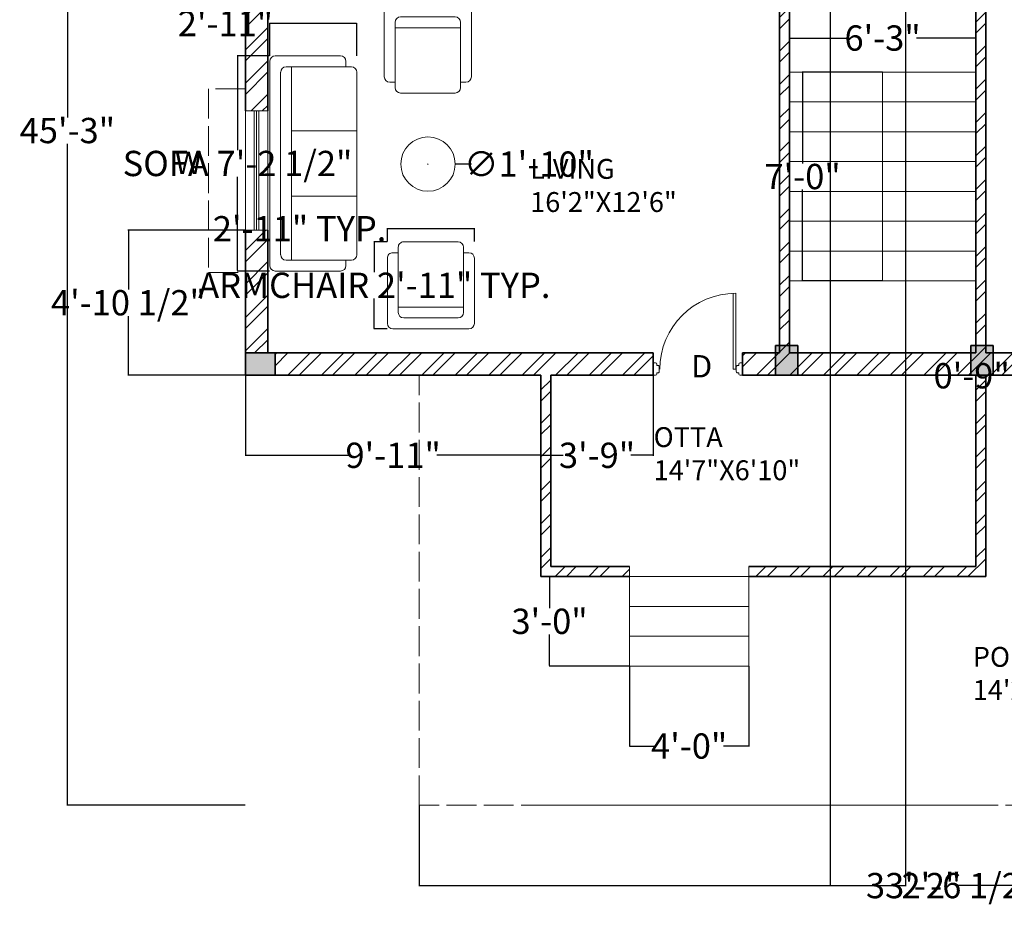
# Model space of a CAD drawing. Units: inches. Extents: x 2379 to 3013, y 1431 to 2110.
# Tile 1 of 10: x 2379 to 2775, y 1431 to 1795. Entities that reach past the tile are written whole.
import ezdxf

# ---------------------------------------------------------------- set-up
doc = ezdxf.new("R2010")
doc.units = ezdxf.units.IN
doc.linetypes.add('ACAD_ISO02W100', pattern=[15, 12, -3])
for name, color, linetype, lineweight in [('00 FURNITURE', 15, 'Continuous', 15), ('A-ANNO-DIMS', 2, 'Continuous', 18), ('A-ANNO-TEXT', 7, 'Continuous', 18), ('A-AREA-IDEN', 7, 'Continuous', 18), ('A-COLS', 7, 'Continuous', 35), ('A-COLS-PATT', 252, 'Continuous', 13), ('A-DOOR', 4, 'Continuous', 18), ('A-FLOR', 8, 'Continuous', 18), ('A-FLOR-STRS', 7, 'Continuous', 18), ('A-ROOF-OVHD', 11, 'ACAD_ISO02W100', 13), ('A-WALL-PATT', 8, 'Continuous', 13), ('WALL', 7, 'Continuous', 35), ('WINDOW', 4, 'Continuous', 15)]:
    doc.layers.add(name, color=color, linetype=linetype, lineweight=lineweight)
doc.styles.get("Standard").update_dxf_attribs({"font": 'arial.ttf'})
doc.dimstyles.get("Standard").update_dxf_attribs({"dimtxt": 10.18, "dimasz": 0.18, "dimexe": 0.18, "dimexo": 0.0625, "dimgap": 0.09, "dimtad": 0, "dimtih": 1, "dimtoh": 1, "dimdec": 0, "dimzin": 0, "dimdsep": 46, "dimlunit": 3, "dimtxsty": 'Standard', "dimcen": 0.09, "dimadec": 0, "dimazin": 0, "dimtfac": 1, "dimtdec": 0, "dimtofl": 0, "dimtmove": 0, "dimatfit": 3, "dimfxl": 1, "dimtolj": 1, "dimtzin": 0, "dimarcsym": 0})

# ---------------------------------------------------------------- blocks, each defined once
blk = doc.blocks.new('column')
for p, q in [((2588.21, 2021.79), (2597.21, 2021.79)), ((2588.21, 2009.79), (2588.21, 2021.79)), ((2597.21, 2021.79), (2597.21, 2009.79)), ((2597.21, 2009.79), (2588.21, 2009.79))]:
    blk.add_line(p, q)
blk = doc.blocks.new('DDD')
at = {"layer": '00 FURNITURE'}
for p, q in [((-12579.77, -15859.53), (-12579.77, -15829.05)), ((-12578.77, -15859.53), (-12578.77, -15829.03)), ((-12612.02, -15857.03), (-12612.02, -15862.03)), ((-12611.02, -15857.03), (-12612.02, -15857.03)), ((-12610.52, -15858.03), (-12610.52, -15857.53)), ((-12578.77, -15859.53), (-12579.77, -15859.53)), ((-12577.52, -15858.03), (-12577.52, -15857.53)), ((-12577.02, -15857.03), (-12576.02, -15857.03)), ((-12576.02, -15857.03), (-12576.02, -15862.03)), ((-12612.02, -15862.03), (-12611.02, -15862.03)), ((-12610.52, -15861.53), (-12610.52, -15861.03)), ((-12577.52, -15861.53), (-12577.52, -15861.03)), ((-12576.02, -15862.03), (-12577.02, -15862.03))]:
    blk.add_line(p, q, dxfattribs=at)
for points in [[(-12610.52, -15861.03), (-12610.02, -15861.03, 0.414214), (-12609.52, -15860.53), (-12609.52, -15858.53, 0.414214), (-12610.02, -15858.03), (-12610.52, -15858.03)], [(-12577.52, -15861.03), (-12578.02, -15861.03, -0.414214), (-12578.52, -15860.53), (-12578.52, -15858.53, -0.414214), (-12578.02, -15858.03), (-12577.52, -15858.03)]]:
    blk.add_lwpolyline(points, format="xyb", dxfattribs=at)
for centre, radius, start, end in [((-12578.77, -15859.53), 30.5, 90, 180), ((-12611.02, -15857.53), 0.5, 0, 90), ((-12577.02, -15857.53), 0.5, 90, 180), ((-12611.02, -15861.53), 0.5, 270, 0), ((-12577.02, -15861.53), 0.5, 180, 270)]:
    blk.add_arc(centre, radius, start, end, dxfattribs=at)
blk = doc.blocks.new('sofa 6')
for p, q in [((-1100, 167), (-1100, 834)), ((-1044, 890), (1044, 890)), ((1100, 834), (1100, 167)), ((-989, 56), (-989, 723)), ((-933, 779), (933, 779)), ((989, 723), (989, 56)), ((-989, 667), (989, 667)), ((-334, 667), (-334, 0)), ((334, 667), (334, 0)), ((-989, 111), (-1044, 111)), ((1044, 111), (989, 111)), ((933, 0), (-933, 0))]:
    blk.add_line(p, q)
for centre, start, end in [((-1044, 834), 90, 180), ((1044, 834), 0, 90), ((-933, 723), 90, 180), ((933, 723), 0, 90), ((-1044, 167), 180, 270), ((1044, 167), 270, 0), ((-933, 56), 180, 270), ((933, 56), 270, 0)]:
    blk.add_arc(centre, 55.6, start, end)
blk = doc.blocks.new('*D12')
at = {"layer": 'A-ANNO-DIMS', "color": 0, "lineweight": -2, "transparency": 16777216}
for p, q in [((2688.63, 1773.67), (2688.63, 1787.52)), ((2763.63, 1773.67), (2763.63, 1787.52)), ((2688.81, 1787.34), (2712.48, 1787.34)), ((2763.45, 1787.34), (2739.78, 1787.34))]:
    blk.add_line(p, q, dxfattribs=at)
at = {"layer": 'A-ANNO-DIMS', "color": 0, "transparency": 16777216}
for points in [[(2688.81, 1787.37), (2688.81, 1787.31), (2688.63, 1787.34)], [(2763.45, 1787.37), (2763.45, 1787.31), (2763.63, 1787.34)]]:
    blk.add_solid(points, dxfattribs=at)
at = {"layer": 'Defpoints', "color": 0, "transparency": 16777216}
for p in [(2763.63, 1787.34), (2688.63, 1773.61), (2763.63, 1773.61)]:
    blk.add_point(p, dxfattribs=at)
at = {"layer": 'A-ANNO-DIMS', "color": 0, "transparency": 16777216, "insert": (2726.13, 1787.34), "char_height": 10.18, "attachment_point": 5}
blk.add_mtext('\\A1;6\'-3"', dxfattribs=at)
blk = doc.blocks.new('*D13')
at = {"layer": 'A-ANNO-DIMS', "color": 0, "lineweight": -2, "transparency": 16777216}
for p, q in [((2469.57, 2021.61), (2397.82, 2021.61)), ((2398, 2021.43), (2398, 1755.4)), ((2398, 1478.79), (2398, 1744.82)), ((2469.57, 1478.61), (2397.82, 1478.61))]:
    blk.add_line(p, q, dxfattribs=at)
at = {"layer": 'A-ANNO-DIMS', "color": 0, "transparency": 16777216}
for points in [[(2397.97, 2021.43), (2398.03, 2021.43), (2398, 2021.61)], [(2397.97, 1478.79), (2398.03, 1478.79), (2398, 1478.61)]]:
    blk.add_solid(points, dxfattribs=at)
at = {"layer": 'Defpoints', "color": 0, "transparency": 16777216}
for p in [(2469.63, 2021.61), (2398, 1478.61), (2469.63, 1478.61)]:
    blk.add_point(p, dxfattribs=at)
at = {"layer": 'A-ANNO-DIMS', "color": 0, "transparency": 16777216, "insert": (2398, 1750.11), "char_height": 10.18, "attachment_point": 5}
blk.add_mtext('\\A1;45\'-3"', dxfattribs=at)
blk = doc.blocks.new('CHAIR-LOUNGE')
for p, q in [((0, 32.85), (0, 6.57)), ((32.85, 35.04), (2.19, 35.04)), ((35.04, 6.57), (35.04, 32.85)), ((4.38, 28.47), (4.38, 2.19)), ((28.47, 30.66), (6.57, 30.66)), ((30.66, 2.19), (30.66, 28.47)), ((30.66, 26.28), (4.38, 26.28)), ((2.19, 4.38), (4.38, 4.38)), ((30.66, 4.38), (32.85, 4.38)), ((6.57, 0), (28.47, 0))]:
    blk.add_line(p, q)
for centre, start, end in [((2.19, 32.85), 90, 180), ((32.85, 32.85), 0, 90), ((6.57, 28.47), 90, 180), ((28.47, 28.47), 0, 90), ((2.19, 6.57), 180, 270), ((32.85, 6.57), 270, 0), ((6.57, 2.19), 180, 270), ((28.47, 2.19), 270, 0)]:
    blk.add_arc(centre, 2.19, start, end)
blk = doc.blocks.new('WIN-48IN')
for p, q in [((0, 48), (0, 0)), ((9, 48), (0, 48)), ((3.5, 48), (3.5, 0)), ((4.5, 48), (4.5, 0)), ((5.5, 48), (5.5, 0)), ((9, 0), (9, 48)), ((9, 0), (0, 0))]:
    blk.add_line(p, q)
blk = doc.blocks.new('*D23')
at = {"layer": 'A-ANNO-DIMS', "color": 0, "lineweight": -2, "transparency": 16777216}
for p, q in [((2816.16, 1660.61), (2808.84, 1660.61)), ((2809.02, 1660.43), (2809.02, 1651.79)), ((2816.16, 1651.61), (2808.84, 1651.61)), ((2809.02, 1651.43), (2808.84, 1651.43)), ((2809.02, 1651.61), (2809.02, 1651.43))]:
    blk.add_line(p, q, dxfattribs=at)
at = {"layer": 'A-ANNO-DIMS', "color": 0, "transparency": 16777216}
for points in [[(2808.99, 1660.43), (2809.05, 1660.43), (2809.02, 1660.61)], [(2808.99, 1651.79), (2809.05, 1651.79), (2809.02, 1651.61)]]:
    blk.add_solid(points, dxfattribs=at)
at = {"layer": 'Defpoints', "color": 0, "transparency": 16777216}
for p in [(2816.22, 1660.61), (2809.02, 1651.61), (2816.22, 1651.61)]:
    blk.add_point(p, dxfattribs=at)
at = {"layer": 'A-ANNO-DIMS', "color": 0, "transparency": 16777216, "insert": (2777.72, 1651.43), "char_height": 10.18, "attachment_point": 5}
blk.add_mtext('\\A1;0\'-9" TYP.', dxfattribs=at)
blk = doc.blocks.new('*D34')
at = {"layer": 'A-ANNO-DIMS', "color": 0, "lineweight": -2, "transparency": 16777216}
for p, q in [((2526.74, 1705.34), (2521.37, 1705.34)), ((2521.55, 1705.16), (2521.55, 1693.18)), ((2521.55, 1670.49), (2521.55, 1682.47)), ((2526.74, 1670.31), (2521.37, 1670.31))]:
    blk.add_line(p, q, dxfattribs=at)
at = {"layer": 'A-ANNO-DIMS', "color": 0, "transparency": 16777216}
for points in [[(2521.52, 1705.16), (2521.58, 1705.16), (2521.55, 1705.34)], [(2521.52, 1670.49), (2521.58, 1670.49), (2521.55, 1670.31)]]:
    blk.add_solid(points, dxfattribs=at)
at = {"layer": 'Defpoints', "color": 0, "transparency": 16777216}
for p in [(2526.81, 1705.34), (2521.55, 1670.31), (2526.81, 1670.31)]:
    blk.add_point(p, dxfattribs=at)
at = {"layer": 'A-ANNO-DIMS', "color": 0, "transparency": 16777216, "insert": (2521.55, 1687.83), "char_height": 10.18, "attachment_point": 5}
blk.add_mtext('\\A1;ARMCHAIR 2\'-11" TYP.', dxfattribs=at)
blk = doc.blocks.new('*D35')
at = {"layer": 'A-ANNO-DIMS', "color": 0, "lineweight": -2, "transparency": 16777216}
for p, q in [((2526.81, 1710.6), (2526.63, 1710.6)), ((2526.81, 1705.41), (2526.81, 1710.78)), ((2561.66, 1710.6), (2526.99, 1710.6)), ((2561.84, 1705.41), (2561.84, 1710.78))]:
    blk.add_line(p, q, dxfattribs=at)
at = {"layer": 'A-ANNO-DIMS', "color": 0, "transparency": 16777216}
for points in [[(2526.99, 1710.63), (2526.99, 1710.57), (2526.81, 1710.6)], [(2561.66, 1710.63), (2561.66, 1710.57), (2561.84, 1710.6)]]:
    blk.add_solid(points, dxfattribs=at)
at = {"layer": 'Defpoints', "color": 0, "transparency": 16777216}
for p in [(2526.81, 1710.6), (2526.81, 1705.34), (2561.84, 1705.34)]:
    blk.add_point(p, dxfattribs=at)
at = {"layer": 'A-ANNO-DIMS', "color": 0, "transparency": 16777216, "insert": (2491.47, 1710.6), "char_height": 10.18, "attachment_point": 5}
blk.add_mtext('\\A1;2\'-11" TYP.', dxfattribs=at)
blk = doc.blocks.new('*D36')
at = {"layer": 'A-ANNO-DIMS', "color": 0, "lineweight": -2, "transparency": 16777216}
for p, q in [((2479.41, 1780.16), (2466.3, 1780.16)), ((2466.48, 1779.98), (2466.48, 1742.21)), ((2466.48, 1693.73), (2466.48, 1731.5)), ((2479.41, 1693.55), (2466.3, 1693.55))]:
    blk.add_line(p, q, dxfattribs=at)
at = {"layer": 'A-ANNO-DIMS', "color": 0, "transparency": 16777216}
for points in [[(2466.45, 1779.98), (2466.51, 1779.98), (2466.48, 1780.16)], [(2466.45, 1693.73), (2466.51, 1693.73), (2466.48, 1693.55)]]:
    blk.add_solid(points, dxfattribs=at)
at = {"layer": 'Defpoints', "color": 0, "transparency": 16777216}
for p in [(2479.47, 1780.16), (2466.48, 1693.55), (2479.47, 1693.55)]:
    blk.add_point(p, dxfattribs=at)
at = {"layer": 'A-ANNO-DIMS', "color": 0, "transparency": 16777216, "insert": (2466.48, 1736.86), "char_height": 10.18, "attachment_point": 5}
blk.add_mtext('\\A1;SOFA 7\'-2 1/2"', dxfattribs=at)
blk = doc.blocks.new('*D37')
at = {"layer": 'A-ANNO-DIMS', "color": 0, "lineweight": -2, "transparency": 16777216}
for p, q in [((2479.47, 1793.16), (2479.29, 1793.16)), ((2479.47, 1780.23), (2479.47, 1793.34)), ((2514.33, 1793.16), (2479.65, 1793.16)), ((2514.51, 1780.23), (2514.51, 1793.34))]:
    blk.add_line(p, q, dxfattribs=at)
at = {"layer": 'A-ANNO-DIMS', "color": 0, "transparency": 16777216}
for points in [[(2479.65, 1793.19), (2479.65, 1793.13), (2479.47, 1793.16)], [(2514.33, 1793.19), (2514.33, 1793.13), (2514.51, 1793.16)]]:
    blk.add_solid(points, dxfattribs=at)
at = {"layer": 'Defpoints', "color": 0, "transparency": 16777216}
for p in [(2479.47, 1793.16), (2479.47, 1780.16), (2514.51, 1780.16)]:
    blk.add_point(p, dxfattribs=at)
at = {"layer": 'A-ANNO-DIMS', "color": 0, "transparency": 16777216, "insert": (2461.63, 1793.16), "char_height": 10.18, "attachment_point": 5}
blk.add_mtext('\\A1;2\'-11"', dxfattribs=at)
blk = doc.blocks.new('*D48')
at = {"layer": 'A-ANNO-DIMS', "color": 0, "lineweight": -2, "transparency": 16777216}
for p, q in [((2624.28, 1534.55), (2624.28, 1502.23)), ((2672.28, 1534.55), (2672.28, 1502.23)), ((2624.46, 1502.41), (2634.46, 1502.41)), ((2672.1, 1502.41), (2662.11, 1502.41))]:
    blk.add_line(p, q, dxfattribs=at)
at = {"layer": 'A-ANNO-DIMS', "color": 0, "transparency": 16777216}
for points in [[(2624.46, 1502.44), (2624.46, 1502.38), (2624.28, 1502.41)], [(2672.1, 1502.44), (2672.1, 1502.38), (2672.28, 1502.41)]]:
    blk.add_solid(points, dxfattribs=at)
at = {"layer": 'Defpoints', "color": 0, "transparency": 16777216}
for p in [(2624.28, 1534.61), (2672.28, 1534.61), (2624.28, 1502.41)]:
    blk.add_point(p, dxfattribs=at)
at = {"layer": 'A-ANNO-DIMS', "color": 0, "transparency": 16777216, "insert": (2648.28, 1502.41), "char_height": 10.18, "attachment_point": 5}
blk.add_mtext('\\A1;4\'-0"', dxfattribs=at)
blk = doc.blocks.new('*D49')
at = {"layer": 'A-ANNO-DIMS', "color": 0, "lineweight": -2, "transparency": 16777216}
for p, q in [((2624.22, 1570.61), (2591.9, 1570.61)), ((2592.08, 1570.43), (2592.08, 1557.9)), ((2592.08, 1534.79), (2592.08, 1547.32)), ((2624.22, 1534.61), (2591.9, 1534.61))]:
    blk.add_line(p, q, dxfattribs=at)
at = {"layer": 'A-ANNO-DIMS', "color": 0, "transparency": 16777216}
for points in [[(2592.05, 1570.43), (2592.11, 1570.43), (2592.08, 1570.61)], [(2592.05, 1534.79), (2592.11, 1534.79), (2592.08, 1534.61)]]:
    blk.add_solid(points, dxfattribs=at)
at = {"layer": 'Defpoints', "color": 0, "transparency": 16777216}
for p in [(2592.08, 1570.61), (2624.28, 1570.61), (2624.28, 1534.61)]:
    blk.add_point(p, dxfattribs=at)
at = {"layer": 'A-ANNO-DIMS', "color": 0, "transparency": 16777216, "insert": (2592.08, 1552.61), "char_height": 10.18, "attachment_point": 5}
blk.add_mtext('\\A1;3\'-0"', dxfattribs=at)
blk = doc.blocks.new('*D50')
at = {"layer": 'A-ANNO-DIMS', "color": 0, "lineweight": -2, "transparency": 16777216}
for p, q in [((2469.63, 1651.55), (2469.63, 1619.23)), ((2588.63, 1651.55), (2588.63, 1619.23)), ((2469.81, 1619.41), (2511.55, 1619.41)), ((2588.45, 1619.41), (2546.7, 1619.41))]:
    blk.add_line(p, q, dxfattribs=at)
at = {"layer": 'A-ANNO-DIMS', "color": 0, "transparency": 16777216}
for points in [[(2469.81, 1619.44), (2469.81, 1619.38), (2469.63, 1619.41)], [(2588.45, 1619.44), (2588.45, 1619.38), (2588.63, 1619.41)]]:
    blk.add_solid(points, dxfattribs=at)
at = {"layer": 'Defpoints', "color": 0, "transparency": 16777216}
for p in [(2469.63, 1651.61), (2588.63, 1651.61), (2469.63, 1619.41)]:
    blk.add_point(p, dxfattribs=at)
at = {"layer": 'A-ANNO-DIMS', "color": 0, "transparency": 16777216, "insert": (2529.13, 1619.41), "char_height": 10.18, "attachment_point": 5}
blk.add_mtext('\\A1;9\'-11"', dxfattribs=at)
blk = doc.blocks.new('*D53')
at = {"layer": 'A-ANNO-DIMS', "color": 0, "lineweight": -2, "transparency": 16777216}
for p, q in [((2704.97, 1871.8), (2704.97, 1446.07)), ((2735.32, 1871.8), (2735.32, 1446.07)), ((2705.15, 1446.25), (2735.14, 1446.25)), ((2735.32, 1446.25), (2735.5, 1446.25))]:
    blk.add_line(p, q, dxfattribs=at)
at = {"layer": 'A-ANNO-DIMS', "color": 0, "transparency": 16777216}
for points in [[(2705.15, 1446.28), (2705.15, 1446.22), (2704.97, 1446.25)], [(2735.14, 1446.28), (2735.14, 1446.22), (2735.32, 1446.25)]]:
    blk.add_solid(points, dxfattribs=at)
at = {"layer": 'Defpoints', "color": 0, "transparency": 16777216}
for p in [(2704.97, 1871.87), (2735.32, 1871.87), (2735.32, 1446.25)]:
    blk.add_point(p, dxfattribs=at)
at = {"layer": 'A-ANNO-DIMS', "color": 0, "transparency": 16777216, "insert": (2761.07, 1446.25), "char_height": 10.18, "attachment_point": 5}
blk.add_mtext('\\A1;2\'-6 1/2"', dxfattribs=at)
blk = doc.blocks.new('*D57')
at = {"layer": 'A-ANNO-DIMS', "color": 0, "lineweight": -2, "transparency": 16777216}
for p, q in [((2469.57, 1710.04), (2422.39, 1710.04)), ((2422.57, 1709.86), (2422.57, 1686.18)), ((2422.57, 1651.79), (2422.57, 1675.47)), ((2469.57, 1651.61), (2422.39, 1651.61))]:
    blk.add_line(p, q, dxfattribs=at)
at = {"layer": 'A-ANNO-DIMS', "color": 0, "transparency": 16777216}
for points in [[(2422.54, 1709.86), (2422.6, 1709.86), (2422.57, 1710.04)], [(2422.54, 1651.79), (2422.6, 1651.79), (2422.57, 1651.61)]]:
    blk.add_solid(points, dxfattribs=at)
at = {"layer": 'Defpoints', "color": 0, "transparency": 16777216}
for p in [(2422.57, 1710.04), (2469.63, 1710.04), (2469.63, 1651.61)]:
    blk.add_point(p, dxfattribs=at)
at = {"layer": 'A-ANNO-DIMS', "color": 0, "transparency": 16777216, "insert": (2422.57, 1680.82), "char_height": 10.18, "attachment_point": 5}
blk.add_mtext('\\A1;4\'-10 1/2"', dxfattribs=at)
blk = doc.blocks.new('*D64')
at = {"layer": 'A-ANNO-DIMS', "color": 0, "lineweight": -2, "transparency": 16777216}
for p, q in [((2588.63, 1651.55), (2588.63, 1619.23)), ((2633.75, 1651.55), (2633.75, 1619.23)), ((2588.81, 1619.41), (2597.57, 1619.41)), ((2633.57, 1619.41), (2624.81, 1619.41))]:
    blk.add_line(p, q, dxfattribs=at)
at = {"layer": 'A-ANNO-DIMS', "color": 0, "transparency": 16777216}
for points in [[(2588.81, 1619.44), (2588.81, 1619.38), (2588.63, 1619.41)], [(2633.57, 1619.44), (2633.57, 1619.38), (2633.75, 1619.41)]]:
    blk.add_solid(points, dxfattribs=at)
at = {"layer": 'Defpoints', "color": 0, "transparency": 16777216}
for p in [(2588.63, 1651.61), (2633.75, 1651.61), (2588.63, 1619.41)]:
    blk.add_point(p, dxfattribs=at)
at = {"layer": 'A-ANNO-DIMS', "color": 0, "transparency": 16777216, "insert": (2611.19, 1619.41), "char_height": 10.18, "attachment_point": 5}
blk.add_mtext('\\A1;3\'-9"', dxfattribs=at)
blk = doc.blocks.new('*D69')
at = {"layer": 'A-ANNO-DIMS', "color": 0, "lineweight": -2, "transparency": 16777216}
for p, q in [((2539.63, 1478.55), (2539.63, 1446.07)), ((2937.63, 1478.55), (2937.63, 1446.07)), ((2539.81, 1446.25), (2721.06, 1446.25)), ((2937.45, 1446.25), (2756.2, 1446.25))]:
    blk.add_line(p, q, dxfattribs=at)
at = {"layer": 'A-ANNO-DIMS', "color": 0, "transparency": 16777216}
for points in [[(2539.81, 1446.28), (2539.81, 1446.22), (2539.63, 1446.25)], [(2937.45, 1446.28), (2937.45, 1446.22), (2937.63, 1446.25)]]:
    blk.add_solid(points, dxfattribs=at)
at = {"layer": 'Defpoints', "color": 0, "transparency": 16777216}
for p in [(2539.63, 1478.61), (2937.63, 1478.61), (2937.63, 1446.25)]:
    blk.add_point(p, dxfattribs=at)
at = {"layer": 'A-ANNO-DIMS', "color": 0, "transparency": 16777216, "insert": (2738.63, 1446.25), "char_height": 10.18, "attachment_point": 5}
blk.add_mtext('\\A1;33\'-2"', dxfattribs=at)
blk = doc.blocks.new('*D71')
at = {"layer": 'A-ANNO-DIMS', "color": 0, "lineweight": -2, "transparency": 16777216}
for p, q in [((2726.07, 1773.61), (2693.75, 1773.61)), ((2693.93, 1773.43), (2693.93, 1736.9)), ((2693.93, 1689.79), (2693.93, 1726.32)), ((2726.07, 1689.61), (2693.75, 1689.61))]:
    blk.add_line(p, q, dxfattribs=at)
at = {"layer": 'A-ANNO-DIMS', "color": 0, "transparency": 16777216}
for points in [[(2693.9, 1773.43), (2693.96, 1773.43), (2693.93, 1773.61)], [(2693.9, 1689.79), (2693.96, 1689.79), (2693.93, 1689.61)]]:
    blk.add_solid(points, dxfattribs=at)
at = {"layer": 'Defpoints', "color": 0, "transparency": 16777216}
for p in [(2693.93, 1773.61), (2726.13, 1773.61), (2726.13, 1689.61)]:
    blk.add_point(p, dxfattribs=at)
at = {"layer": 'A-ANNO-DIMS', "color": 0, "transparency": 16777216, "insert": (2693.93, 1731.61), "char_height": 10.18, "attachment_point": 5}
blk.add_mtext('\\A1;7\'-0"', dxfattribs=at)
blk = doc.blocks.new('*D72')
at = {"layer": 'A-ANNO-DIMS', "color": 0, "lineweight": -2, "transparency": 16777216}
for p, q in [((2543.06, 1736.61), (2543.24, 1736.61)), ((2543.15, 1736.52), (2543.15, 1736.7)), ((2560.67, 1736.61), (2554.28, 1736.61))]:
    blk.add_line(p, q, dxfattribs=at)
at = {"layer": 'A-ANNO-DIMS', "color": 0, "transparency": 16777216}
blk.add_solid([(2554.28, 1736.64), (2554.28, 1736.58), (2554.1, 1736.61)], dxfattribs=at)
at = {"layer": 'Defpoints', "color": 0, "transparency": 16777216}
for p in [(2532.2, 1736.61), (2554.1, 1736.61)]:
    blk.add_point(p, dxfattribs=at)
at = {"layer": 'A-ANNO-DIMS', "color": 0, "transparency": 16777216, "insert": (2583.79, 1736.61), "char_height": 10.18, "attachment_point": 5}
blk.add_mtext('\\A1;∅1\'-10"', dxfattribs=at)

msp = doc.modelspace()

# ---------------------------------------------------------------- hatches: boundary and pattern name
at = {"layer": 'A-COLS-PATT'}
h = msp.add_hatch(color=256, dxfattribs=at)
h.dxf.hatch_style = 1
h.paths.add_polyline_path([(2937.62, 1660.61), (2925.62, 1660.61), (2925.62, 1651.61), (2937.62, 1651.61)])
h.paths.add_polyline_path([(2481.63, 1809.61), (2478.63, 1809.61), (2478.63, 1811.02), (2469.63, 1811.02), (2469.63, 1802.02), (2478.63, 1802.02), (2478.63, 1805.61), (2481.63, 1805.61)])
h.paths.add_polyline_path([(2481.63, 1811.02), (2478.63, 1811.02), (2478.63, 1809.61), (2481.63, 1809.61)], flags=17)
h.paths.add_polyline_path([(2481.63, 1805.61), (2478.63, 1805.61), (2478.63, 1802.02), (2481.63, 1802.02)], flags=17)
h.paths.add_polyline_path([(2481.63, 1660.61), (2469.63, 1660.61), (2469.63, 1651.61), (2481.63, 1651.61)])
h.paths.add_polyline_path([(2692.07, 1660.61), (2688.63, 1660.61), (2688.63, 1663.61), (2684.63, 1663.61), (2684.63, 1660.61), (2683.07, 1660.61), (2683.07, 1651.61), (2692.07, 1651.61)])
h.paths.add_polyline_path([(2692.07, 1663.61), (2688.63, 1663.61), (2688.63, 1660.61), (2692.07, 1660.61)], flags=17)
h.paths.add_polyline_path([(2684.63, 1663.61), (2683.07, 1663.61), (2683.07, 1660.61), (2684.63, 1660.61)], flags=17)
h.paths.add_polyline_path([(2770.63, 1660.61), (2767.63, 1660.61), (2767.63, 1663.61), (2763.63, 1663.61), (2763.63, 1660.61), (2761.63, 1660.61), (2761.63, 1651.61), (2763.63, 1651.61), (2767.63, 1651.61), (2767.63, 1651.61), (2770.63, 1651.61)])
h.paths.add_polyline_path([(2770.63, 1663.61), (2767.63, 1663.61), (2767.63, 1660.61), (2770.63, 1660.61)], flags=17)
h.paths.add_polyline_path([(2763.63, 1663.61), (2761.63, 1663.61), (2761.63, 1660.61), (2763.63, 1660.61)], flags=17)
h.paths.add_polyline_path([(2937.63, 1813.62), (2928.63, 1813.62), (2928.63, 1810.61), (2925.63, 1810.61), (2925.63, 1806.61), (2928.63, 1806.61), (2928.63, 1804.62), (2937.63, 1804.62)], flags=17)
h.paths.add_polyline_path([(2937.63, 1813.62), (2928.63, 1813.62), (2928.63, 1810.61), (2925.63, 1810.61), (2925.63, 1804.62), (2937.63, 1804.62)], flags=17)
h.paths.add_polyline_path([(2928.63, 1813.62), (2925.63, 1813.62), (2925.63, 1810.61), (2928.63, 1810.61)], flags=0)
h.paths.add_polyline_path([(2937.63, 1863.8), (2928.63, 1863.8), (2928.63, 1862.61), (2925.63, 1862.61), (2925.63, 1858.61), (2928.63, 1858.61), (2928.63, 1854.8), (2937.63, 1854.8)])
h.paths.add_polyline_path([(2928.63, 1863.8), (2925.63, 1863.8), (2925.63, 1862.61), (2928.63, 1862.61)], flags=17)
h.paths.add_polyline_path([(2928.63, 1858.61), (2925.63, 1858.61), (2925.63, 1854.8), (2928.63, 1854.8)], flags=17)
h.paths.add_polyline_path([(2937.63, 2021.61), (2928.63, 2021.61), (2928.63, 2012.61), (2928.63, 2012.61), (2928.63, 2009.61), (2937.63, 2009.61)])
h.paths.add_polyline_path([(2770.27, 2021.61), (2761.27, 2021.61), (2761.27, 2012.61), (2763.63, 2012.61), (2763.63, 2009.61), (2767.63, 2009.61), (2767.63, 2012.61), (2770.27, 2012.61)])
h.paths.add_polyline_path([(2763.63, 2012.61), (2761.27, 2012.61), (2761.27, 2009.61), (2763.63, 2009.61)], flags=17)
h.paths.add_polyline_path([(2770.27, 2012.61), (2767.63, 2012.61), (2767.63, 2009.61), (2770.27, 2009.61)], flags=17)
h.paths.add_polyline_path([(2597.21, 2021.61), (2588.21, 2021.61), (2588.21, 2012.61), (2590.63, 2012.61), (2590.63, 2009.61), (2594.63, 2009.61), (2594.63, 2012.61), (2597.21, 2012.61)])
h.paths.add_polyline_path([(2590.63, 2012.61), (2588.21, 2012.61), (2588.21, 2009.61), (2590.63, 2009.61)], flags=17)
h.paths.add_polyline_path([(2597.21, 2012.61), (2594.63, 2012.61), (2594.63, 2009.61), (2597.21, 2009.61)], flags=17)
at = {"layer": 'A-WALL-PATT'}
h = msp.add_hatch(dxfattribs=at)
h.set_pattern_fill('ANSI32', color=256)
h.paths.add_polyline_path([(2925.63, 1862.61), (2815.63, 1862.61), (2815.63, 1858.61), (2827.63, 1858.61), (2827.63, 1810.61), (2815.63, 1810.61), (2815.63, 1806.61), (2850.78, 1806.61), (2850.78, 1810.61), (2831.63, 1810.61), (2831.63, 1858.61), (2925.63, 1858.61)])
h.paths.add_polyline_path([(2925.63, 1810.61), (2880.78, 1810.61), (2880.78, 1806.61), (2925.63, 1806.61)], flags=17)
h.paths.add_polyline_path([(2633.75, 1660.61), (2594.63, 1660.61), (2481.63, 1660.61), (2481.63, 1651.61), (2588.63, 1651.61), (2588.63, 1570.61), (2624.28, 1570.61), (2624.28, 1574.61), (2592.63, 1574.61), (2592.63, 1651.61), (2633.75, 1651.61)])
h.paths.add_polyline_path([(2594.63, 1809.61), (2481.63, 1809.61), (2481.63, 1805.61), (2594.63, 1805.61)])
h.paths.add_polyline_path([(2594.63, 2012.61), (2597.21, 2012.61), (2597.21, 2021.61), (2588.21, 2021.61), (2588.21, 2012.61), (2590.63, 2012.61), (2590.63, 1845.61), (2594.63, 1845.61)])
h.paths.add_polyline_path([(2767.63, 2012.61), (2770.27, 2012.61), (2770.27, 2021.61), (2761.27, 2021.61), (2761.27, 2012.61), (2763.63, 2012.61), (2763.63, 1928.61), (2691.63, 1928.61), (2643.63, 1928.61), (2643.63, 1924.61), (2691.63, 1924.61), (2763.63, 1924.61), (2763.63, 1858.61), (2779.63, 1858.61), (2779.63, 1862.61), (2767.63, 1862.61)])
h.paths.add_polyline_path([(2613.63, 2012.61), (2613.63, 2021.61), (2597.21, 2021.61), (2597.21, 2012.61)])
h.paths.add_polyline_path([(2508.33, 2012.61), (2508.33, 2021.61), (2478.63, 2021.61), (2478.63, 2012.61)])
h.paths.add_polyline_path([(2556.33, 2021.61), (2556.33, 2012.61), (2588.21, 2012.61), (2588.21, 2021.61)])
h.paths.add_polyline_path([(2659.15, 2012.61), (2659.15, 2021.61), (2643.63, 2021.61), (2643.63, 1958.61), (2661.63, 1958.61), (2661.63, 1962.61), (2647.63, 1962.61), (2647.63, 2012.61)])
h.paths.add_polyline_path([(2714.17, 2012.61), (2714.17, 2021.61), (2683.15, 2021.61), (2683.15, 2012.61), (2691.63, 2012.61), (2691.63, 1958.61), (2695.63, 1958.61), (2695.63, 2012.61)])
h.paths.add_polyline_path([(2738.17, 2021.61), (2738.17, 2012.61), (2761.27, 2012.61), (2761.27, 2021.61)])
h.paths.add_polyline_path([(2820.76, 2012.61), (2820.76, 2021.61), (2770.27, 2021.61), (2770.27, 2012.61)])
h.paths.add_polyline_path([(2868.76, 2021.61), (2868.76, 2012.61), (2928.63, 2012.61), (2928.63, 2021.61)])
h.paths.add_polyline_path([(2928.63, 1962.9), (2937.63, 1962.9), (2937.63, 2009.61), (2928.63, 2009.61)])
h.paths.add_polyline_path([(2937.63, 1914.9), (2928.63, 1914.9), (2928.63, 1863.8), (2937.63, 1863.8)])
h.paths.add_polyline_path([(2928.63, 1846.59), (2937.63, 1846.59), (2937.63, 1854.8), (2928.63, 1854.8)])
h.paths.add_polyline_path([(2937.63, 1822.59), (2928.63, 1822.59), (2928.63, 1813.62), (2937.63, 1813.62)])
h.paths.add_polyline_path([(2928.63, 1778.48), (2937.63, 1778.48), (2937.63, 1813.62), (2928.63, 1813.62), (2928.63, 1810.61), (2925.63, 1810.61), (2925.63, 1806.61), (2928.63, 1806.61)])
h.paths.add_polyline_path([(2816.22, 1651.61), (2816.22, 1660.61), (2767.63, 1660.61), (2767.63, 1806.61), (2779.63, 1806.61), (2779.63, 1810.61), (2763.63, 1810.61), (2763.63, 1660.61), (2688.63, 1660.61), (2688.63, 1810.61), (2684.63, 1810.61), (2684.63, 1660.61), (2669.75, 1660.61), (2669.75, 1651.61), (2763.63, 1651.61), (2763.63, 1574.61), (2672.28, 1574.61), (2672.28, 1570.61), (2767.63, 1570.61), (2767.63, 1651.61)])
h.paths.add_polyline_path([(2864.22, 1660.61), (2864.22, 1651.61), (2937.63, 1651.61), (2937.63, 1730.48), (2928.63, 1730.48), (2928.63, 1660.61)])
h.paths.add_polyline_path([(2469.63, 1975.19), (2478.63, 1975.19), (2478.63, 2009.61), (2469.63, 2009.61)])
h.paths.add_polyline_path([(2478.63, 1927.19), (2469.63, 1927.19), (2469.63, 1811.02), (2478.63, 1811.02)])
h.paths.add_polyline_path([(2469.63, 1758.04), (2478.63, 1758.04), (2478.63, 1802.02), (2469.63, 1802.02)])
h.paths.add_polyline_path([(2478.63, 1710.04), (2469.63, 1710.04), (2469.63, 1660.61), (2478.63, 1660.61)])

# ---------------------------------------------------------------- linework, layer by layer
at = {"layer": '00 FURNITURE'}
msp.add_circle((2543.15, 1736.61), 10.95, dxfattribs=at)
at = {"layer": 'A-FLOR'}
msp.add_line((2588.63, 1478.61), (2767.63, 1478.61), dxfattribs=at)
at = {"layer": 'A-FLOR-STRS'}
for p, q in [((2688.63, 1773.61), (2763.63, 1773.61)), ((2726.13, 1689.61), (2726.13, 1773.61)), ((2688.63, 1761.61), (2763.63, 1761.61)), ((2688.63, 1749.61), (2763.63, 1749.61)), ((2688.63, 1737.61), (2763.63, 1737.61)), ((2688.63, 1725.61), (2763.63, 1725.61)), ((2688.63, 1713.61), (2763.63, 1713.61)), ((2688.63, 1701.61), (2763.63, 1701.61)), ((2688.63, 1689.61), (2763.63, 1689.61)), ((2624.28, 1574.61), (2624.28, 1534.61)), ((2672.28, 1574.61), (2672.28, 1534.61)), ((2624.28, 1570.61), (2672.28, 1570.61)), ((2624.28, 1558.61), (2672.28, 1558.61)), ((2624.28, 1546.61), (2672.28, 1546.61)), ((2624.28, 1534.61), (2672.28, 1534.61))]:
    msp.add_line(p, q, dxfattribs=at)
at = {"layer": 'A-ROOF-OVHD'}
for p, q in [((2469.63, 1766.94), (2454.77, 1766.94)), ((2454.77, 1766.94), (2454.77, 1692.99)), ((2454.77, 1692.99), (2469.63, 1692.99)), ((2539.63, 1478.61), (2539.63, 1651.61)), ((2937.63, 1478.61), (2539.63, 1478.61))]:
    msp.add_line(p, q, dxfattribs=at)
at = {"layer": 'WALL'}
for p, q in [((2469.63, 1758.04), (2469.63, 1927.19)), ((2684.63, 1810.61), (2684.63, 1660.61)), ((2688.63, 1810.61), (2688.63, 1660.61)), ((2763.63, 1810.61), (2763.63, 1660.61)), ((2478.63, 1758.04), (2478.63, 1805.61)), ((2767.63, 1806.61), (2767.63, 1660.61)), ((2469.63, 1651.61), (2469.63, 1710.04)), ((2478.63, 1660.61), (2478.63, 1710.04)), ((2478.63, 1660.61), (2594.63, 1660.61)), ((2594.63, 1660.61), (2633.75, 1660.61)), ((2633.75, 1651.61), (2633.75, 1660.61)), ((2669.75, 1651.61), (2669.75, 1660.61)), ((2669.75, 1660.61), (2684.63, 1660.61)), ((2688.63, 1660.61), (2763.63, 1660.61)), ((2767.63, 1660.61), (2816.22, 1660.61)), ((2469.63, 1651.61), (2588.63, 1651.61)), ((2469.63, 1651.61), (2588.63, 1651.61)), ((2588.63, 1651.61), (2588.63, 1570.61)), ((2592.63, 1651.61), (2592.63, 1574.61)), ((2592.63, 1651.61), (2633.75, 1651.61)), ((2592.63, 1651.61), (2633.75, 1651.61)), ((2669.75, 1651.61), (2763.63, 1651.61)), ((2669.75, 1651.61), (2763.63, 1651.61)), ((2763.63, 1651.61), (2763.63, 1574.61)), ((2767.63, 1651.61), (2767.63, 1570.61)), ((2767.63, 1651.61), (2816.22, 1651.61)), ((2592.63, 1574.61), (2624.28, 1574.61)), ((2672.28, 1574.61), (2763.63, 1574.61)), ((2588.63, 1570.61), (2624.28, 1570.61)), ((2672.28, 1570.61), (2767.63, 1570.61))]:
    msp.add_line(p, q, dxfattribs=at)

# ---------------------------------------------------------------- block references
at = {"layer": '00 FURNITURE'}
msp.add_blockref('CHAIR-LOUNGE', (2525.56, 1765.19), dxfattribs=at)
at = {"layer": '00 FURNITURE', "xscale": -0.0393700787401575, "yscale": 0.0393700787401575, "zscale": 0.0393700787401575, "rotation": 90}
msp.add_blockref('sofa 6', (2514.51, 1736.86), dxfattribs=at)
at = {"layer": '00 FURNITURE', "rotation": 180}
msp.add_blockref('CHAIR-LOUNGE', (2561.84, 1705.34), dxfattribs=at)
at = {"layer": 'A-COLS'}
for p, rotation in [((459.84, 4248.82), 270), ((5280.29, 3673.4), 180), ((5358.84, 3673.4), 180)]:
    msp.add_blockref('column', p, dxfattribs=dict(at, rotation=rotation))
at = {"layer": 'A-DOOR'}
msp.add_blockref('DDD', (15245.78, 17513.64), dxfattribs=at)
at = {"layer": 'WINDOW', "rotation": 359.9999987925818}
msp.add_blockref('WIN-48IN', (2469.63, 1710.04), dxfattribs=at)

# ---------------------------------------------------------------- texts
at = {"layer": 'A-ANNO-TEXT', "char_height": 9, "attachment_point": 1}
for s, insert in [('W', (2441.31, 1741.56)), ('D', (2649.1, 1659.74))]:
    msp.add_mtext_dynamic_manual_height_columns(s, width=106.8919, gutter_width=12.5, heights=[0], dxfattribs=dict(at, insert=insert))
at = {"layer": 'A-AREA-IDEN', "char_height": 8, "attachment_point": 1}
for s, insert in [('LIVING\\P16\'2"X12\'6"                  ', (2584.29, 1738.68)), ('OTTA\\P14\'7"X6\'10"  ', (2633.97, 1630.73)), ('PORCH\\P14\'2"X12\'3"               ', (2762.44, 1542.3))]:
    msp.add_mtext_dynamic_manual_height_columns(s, width=46.1506, gutter_width=12.5, heights=[0], dxfattribs=dict(at, insert=insert))

# ---------------------------------------------------------------- dimensions: what is measured, and where the dimension line sits
at = {"layer": 'A-ANNO-DIMS'}
for base, p1, p2, angle, override, picture, middle in [((2398, 1478.61), (2469.63, 2021.61), (2469.63, 1478.61), 90, {"dimclrd": 0, "dimclre": 0, "dimclrt": 0}, '*D13', (2398, 1750.11)), ((2479.47, 1793.16), (2514.51, 1780.16), (2479.47, 1780.16), 180, {"dimdec": 1, "dimlfac": 1, "dimrnd": 0, "dimzin": 1, "dimdsep": 46, "dimlunit": 4, "dimfrac": 2}, '*D37', (2461.63, 1793.16)), ((2693.93, 1773.61), (2726.13, 1689.61), (2726.13, 1773.61), 90, {"dimdec": 1, "dimlfac": 1, "dimrnd": 0, "dimzin": 1, "dimdsep": 46, "dimlunit": 4, "dimfrac": 2}, '*D71', (2693.93, 1731.61)), ((2422.57, 1710.04), (2469.63, 1651.61), (2469.63, 1710.04), 90, {"dimdec": 1, "dimlfac": 1, "dimrnd": 0, "dimzin": 1, "dimdsep": 46, "dimlunit": 4, "dimfrac": 2}, '*D57', (2422.57, 1680.82)), ((2469.63, 1619.41), (2588.63, 1651.61), (2469.63, 1651.61), 180, {"dimdec": 1, "dimlfac": 1, "dimrnd": 0, "dimzin": 1, "dimdsep": 46, "dimlunit": 4, "dimfrac": 2}, '*D50', (2529.13, 1619.41)), ((2588.63, 1619.41), (2633.75, 1651.61), (2588.63, 1651.61), 180, {"dimdec": 1, "dimlfac": 1, "dimrnd": 0, "dimzin": 1, "dimdsep": 46, "dimlunit": 4, "dimfrac": 2}, '*D64', (2611.19, 1619.41)), ((2592.08, 1570.61), (2624.28, 1534.61), (2624.28, 1570.61), 90, {"dimdec": 1, "dimlfac": 1, "dimrnd": 0, "dimzin": 1, "dimdsep": 46, "dimlunit": 4, "dimfrac": 2}, '*D49', (2592.08, 1552.61)), ((2624.28, 1502.41), (2672.28, 1534.61), (2624.28, 1534.61), 180, {"dimdec": 1, "dimlfac": 1, "dimrnd": 0, "dimzin": 1, "dimdsep": 46, "dimlunit": 4, "dimfrac": 2}, '*D48', (2648.28, 1502.41))]:
    dim = msp.add_linear_dim(base=base, p1=p1, p2=p2, angle=angle, dimstyle='Standard', override=override, dxfattribs=at)
    dim.commit()
    dim.dimension.update_dxf_attribs({"geometry": picture, "text_midpoint": middle})
for base, p1, p2, override, picture, middle in [((2735.3226, 1446.2521), (2704.974, 1871.8654), (2735.3226, 1871.8654), {"dimdec": 1, "dimlfac": 1, "dimrnd": 0, "dimzin": 1, "dimdsep": 46, "dimlunit": 4, "dimfrac": 2}, '*D53', (2761.0704, 1446.2521)), ((2763.63, 1787.34), (2688.63, 1773.61), (2763.63, 1773.61), {"dimclrd": 0, "dimclre": 0, "dimclrt": 0}, '*D12', (2726.13, 1787.34)), ((2937.63, 1446.25), (2539.63, 1478.61), (2937.63, 1478.61), {"dimdec": 1, "dimlfac": 1, "dimrnd": 0, "dimzin": 1, "dimdsep": 46, "dimlunit": 4, "dimfrac": 2}, '*D69', (2738.63, 1446.25))]:
    dim = msp.add_linear_dim(base=base, p1=p1, p2=p2, dimstyle='Standard', override=override, dxfattribs=at)
    dim.commit()
    dim.dimension.update_dxf_attribs({"geometry": picture, "text_midpoint": middle})
for base, p1, p2, angle, text, picture, middle in [((2466.48, 1693.55), (2479.47, 1780.16), (2479.47, 1693.55), 270, 'SOFA <>', '*D36', (2466.48, 1736.86)), ((2526.81, 1710.6), (2561.84, 1705.34), (2526.81, 1705.34), 180, '<> TYP.', '*D35', (2491.47, 1710.6)), ((2521.55, 1670.31), (2526.81, 1705.34), (2526.81, 1670.31), 270, 'ARMCHAIR <> TYP.', '*D34', (2521.55, 1687.83)), ((2809.02, 1651.61), (2816.22, 1660.61), (2816.22, 1651.61), 270, '<> TYP.', '*D23', (2777.72, 1651.43))]:
    dim = msp.add_linear_dim(base=base, p1=p1, p2=p2, angle=angle, text=text, dimstyle='Standard', override={"dimdec": 1, "dimlfac": 1, "dimrnd": 0, "dimzin": 1, "dimdsep": 46, "dimlunit": 4, "dimfrac": 2}, dxfattribs=at)
    dim.commit()
    dim.dimension.update_dxf_attribs({"geometry": picture, "text_midpoint": middle})
dim = msp.add_diameter_dim_2p(p1=(2532.2, 1736.61), p2=(2554.1, 1736.61), dimstyle='Standard', override={"dimdec": 1, "dimlfac": 1, "dimrnd": 0, "dimzin": 1, "dimdsep": 46, "dimlunit": 4, "dimfrac": 2}, dxfattribs=at)
dim.commit()
dim.dimension.update_dxf_attribs({"geometry": '*D72', "text_midpoint": (2560.67, 1736.61), "dimtype": 163})

doc.saveas('drawing.dxf')
